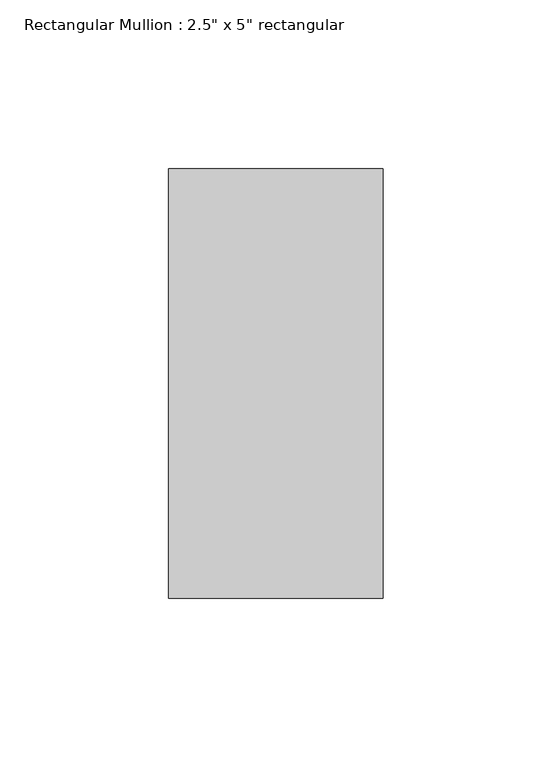
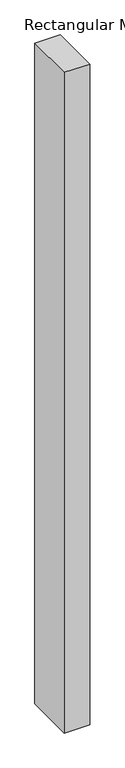
"""IFC4 building model written with IfcOpenShell, lengths in millimetres: member geometry."""

from ifc_helpers import new_model, si_unit, frame, origin, place, context, project, spatial, polyline, outline, extrude, source, transform, mapped, element, save


def member_58157355(model_context):
    return source(origin(), model_context, "Body", "SweptSolid", [
        extrude(outline(polyline([(0.0, 63.5), (0.0, -63.5), (-63.5, -63.5), (-63.5, 63.5), (0.0, 63.5)])), frame((0.0, 0.0, -1745.718644), z_axis=(0.0, 0.0, 1.0), x_axis=(1.0, 0.0, 0.0)), (0.0, 0.0, 1.0), 1745.718644),
    ])


if __name__ == "__main__":
    model = new_model("IFC4")
    model_context = context("Model", 3, world=origin())
    ifc_project = project(units=[si_unit("LENGTHUNIT", "METRE", prefix="MILLI")], contexts=[model_context])
    site = spatial("IfcSite", under=ifc_project)
    building = spatial("IfcBuilding", under=site)
    placement = place(None, origin())
    member_shape = member_58157355(model_context)
    element("IfcMember", 1, ObjectType="Rectangular Mullion : 2.5\" x 5\" rectangular", at=placement, inside=building, context=model_context, shape_type="MappedRepresentation", body=[
        mapped(member_shape, transform((0.0, 0.0, 0.0), x_axis=(1.0, 0.0, 0.0), y_axis=(0.0, 1.0, 0.0), z_axis=(0.0, 0.0, 1.0))),
    ])
    save(model, "model.ifc")

# Revit data of these elements
# Type "Rectangular Mullion : 2.5\" x 5\" rectangular"
#   built-in parameter 1007304 = 0.416667 (stored number, unit not read)
#   built-in parameter 1007301 = 0.104167 (stored number, unit not read)
#   built-in parameter 1007300 = 0.104167 (stored number, unit not read)
# Element 1 (IfcMember, "Rectangular Mullion : 2.5\" x 5\" rectangular")
#   Materials on its faces: "Aluminum"
# Materials
#   "Aluminum": class "Metal", colour RGB 247 247 247, transparency 0, Description = "Aluminum 6061", Cost = 0
